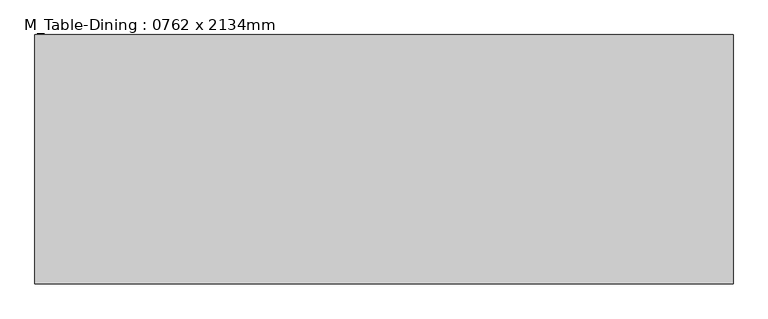
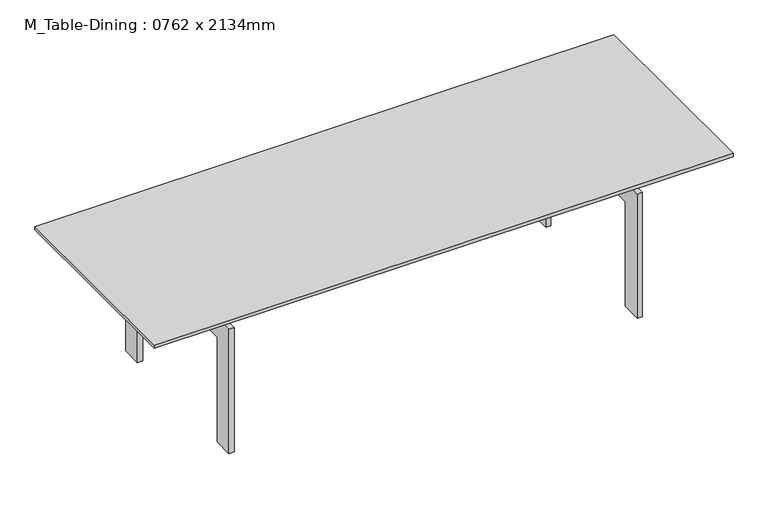
"""IFC4 building model written with IfcOpenShell, lengths in millimetres: furniture geometry, M_Table-Dining : 0762 x 2134mm."""

from ifc_helpers import new_model, si_unit, frame, origin, place, context, project, spatial, polyline, outline, extrude, source, transform, mapped, element, save


def m_table_dining_0762_x_2134mm_3327233b(model_context):
    return source(origin(), model_context, "Body", "SweptSolid", [
        extrude(outline(polyline([(983.6657667, 297.7823857), (983.6657667, 272.3823857), (-947.1342333, 272.3823857), (-947.1342333, 297.7823857), (983.6657667, 297.7823857)])), frame((0.0, 0.0, 483.8), z_axis=(0.0, 0.0, 1.0), x_axis=(1.0, 0.0, 0.0)), (0.0, 0.0, 1.0), 63.5),
        extrude(outline(polyline([(983.6657667, -82.5889222), (983.6657667, -107.9889222), (-947.1342333, -107.9889222), (-947.1342333, -82.5889222), (983.6657667, -82.5889222)])), frame((0.0, 0.0, 483.8), z_axis=(0.0, 0.0, 1.0), x_axis=(1.0, 0.0, 0.0)), (0.0, 0.0, 1.0), 63.5),
        extrude(outline(polyline([(425.4110778, 0.0), (349.2110778, 0.0), (349.2110778, 407.6), (-158.7889222, 407.6), (-158.7889222, 0.0), (-234.9889222, 0.0), (-234.9889222, 483.8), (425.4110778, 483.8), (425.4110778, 0.0)])), frame((761.4157667, 0.0, 0.0), z_axis=(1.0, 0.0, 0.0), x_axis=(0.0, 1.0, 0.0)), (0.0, 0.0, 1.0), 19.05),
        extrude(outline(polyline([(425.4110778, 483.8), (425.4110778, 0.0), (349.2110778, 0.0), (349.2110778, 407.6), (-158.7889222, 407.6), (-158.7889222, 0.0), (-234.9889222, 0.0), (-234.9889222, 483.8), (425.4110778, 483.8)])), frame((-743.9342333, 0.0, 0.0), z_axis=(1.0, 0.0, 0.0), x_axis=(0.0, 1.0, 0.0)), (0.0, 0.0, 1.0), 19.05),
        extrude(outline(polyline([(1085.2657667, 476.2110778), (1085.2657667, -285.7889222), (-1048.7342333, -285.7889222), (-1048.7342333, 476.2110778), (1085.2657667, 476.2110778)])), frame((0.0, 0.0, 547.3), z_axis=(0.0, 0.0, 1.0), x_axis=(1.0, 0.0, 0.0)), (0.0, 0.0, 1.0), 12.7),
    ])


if __name__ == "__main__":
    model = new_model("IFC4")
    model_context = context("Model", 3, world=origin())
    ifc_project = project(units=[si_unit("LENGTHUNIT", "METRE", prefix="MILLI")], contexts=[model_context])
    site = spatial("IfcSite", under=ifc_project)
    building = spatial("IfcBuilding", under=site)
    placement = place(None, origin())
    m_table_dining_0762_x_2134mm_shape = m_table_dining_0762_x_2134mm_3327233b(model_context)
    element("IfcFurniture", 1, ObjectType="M_Table-Dining : 0762 x 2134mm", at=placement, inside=building, context=model_context, shape_type="MappedRepresentation", body=[
        mapped(m_table_dining_0762_x_2134mm_shape, transform((0.0, 0.0, 0.0), x_axis=(1.0, 0.0, 0.0), y_axis=(0.0, 1.0, 0.0), z_axis=(0.0, 0.0, 1.0))),
    ])
    save(model, "model.ifc")

# Revit data of these elements
# Type "M_Table-Dining : 0762 x 2134mm"
#   Height = 560 mm
#   Length = 2134 mm
#   Width = 762 mm
#   Base Material = Steel, Chrome Plated
#   Top Material = Glass - Clear, Grey
#   Default Elevation = 0
# Element 1 (IfcFurniture, "M_Table-Dining : 0762 x 2134mm")
#   Materials on its faces: "Steel, Chrome Plated", "Glass - Clear, Grey"
# Materials
#   "Steel, Chrome Plated": class "Metal", colour RGB 244 244 244, transparency 0, Description = "Chromiuim plated steel", Cost = 0
#   "Glass - Clear, Grey": class "Glass", colour RGB 252 255 255, transparency 0.64
